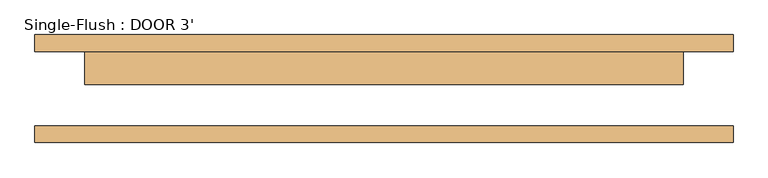
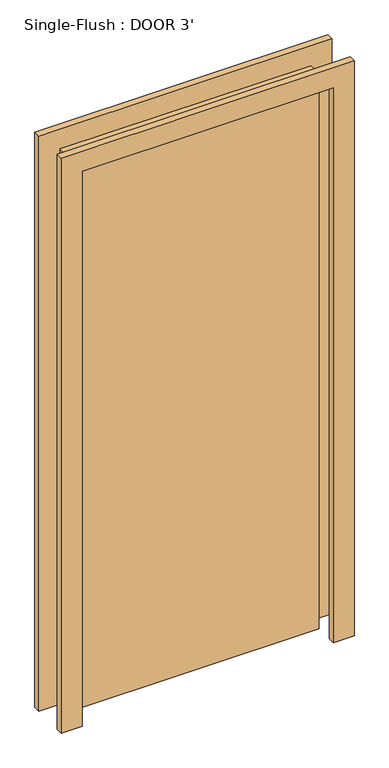
"""IFC4 building model written with IfcOpenShell, lengths in millimetres: door geometry, Single-Flush : DOOR 3'."""

from ifc_helpers import new_model, si_unit, frame, origin, origin_with_axes, place, context, project, spatial, polyline, outline, extrude, source, transform, mapped, element, save


def single_flush_door_3_e5f9f3c4(model_context):
    return source(origin(), model_context, "Body", "SweptSolid", [
        extrude(outline(polyline([(2209.8, -533.4), (0.0, -533.4), (0.0, -457.2), (2133.6, -457.2), (2133.6, 457.2), (0.0, 457.2), (0.0, 533.4), (2209.8, 533.4), (2209.8, -533.4)])), frame((0.0, 57.15, 0.0), z_axis=(0.0, 1.0, 0.0), x_axis=(0.0, 0.0, 1.0)), (0.0, 0.0, 1.0), 25.4),
        extrude(outline(polyline([(2209.8, 533.4), (2209.8, -533.4), (0.0, -533.4), (0.0, -457.2), (2133.6, -457.2), (2133.6, 457.2), (0.0, 457.2), (0.0, 533.4), (2209.8, 533.4)])), frame((0.0, -82.55, 0.0), z_axis=(0.0, 1.0, 0.0), x_axis=(0.0, 0.0, 1.0)), (0.0, 0.0, 1.0), 25.4),
        extrude(outline(polyline([(457.2, 6.35), (-457.2, 6.35), (-457.2, 57.15), (457.2, 57.15), (457.2, 6.35)])), origin_with_axes(), (0.0, 0.0, 1.0), 2133.6),
    ])


if __name__ == "__main__":
    model = new_model("IFC4")
    model_context = context("Model", 3, world=origin())
    ifc_project = project(units=[si_unit("LENGTHUNIT", "METRE", prefix="MILLI")], contexts=[model_context])
    site = spatial("IfcSite", under=ifc_project)
    building = spatial("IfcBuilding", under=site)
    placement = place(None, origin())
    single_flush_door_3_shape = single_flush_door_3_e5f9f3c4(model_context)
    element("IfcDoor", 1, ObjectType="Single-Flush : DOOR 3'", at=placement, inside=building, context=model_context, shape_type="MappedRepresentation", body=[
        mapped(single_flush_door_3_shape, transform((0.0, 0.0, 0.0), x_axis=(1.0, 0.0, 0.0), y_axis=(0.0, 1.0, 0.0), z_axis=(0.0, 0.0, 1.0))),
    ])
    save(model, "model.ifc")

# Revit data of these elements
# Type "Single-Flush : DOOR 3'"
#   Type Mark = "9"
#   Construction Type Id = "MDOOR"
#   Assembly Code = "C1020"
#   Analytic Construction = "Metal"
#   Thickness = 0' - 2"
#   Heat Transfer Coefficient (U) = 0.651978 BTU/(h·ft²·°F)
#   Height = 7' - 0"
#   Trim Projection Ext = 0' - 1"
#   Trim Projection Int = 0' - 1"
#   Trim Width = 0' - 3"
#   Width = 3' - 0"
#   Define Thermal Properties by = 1
#   Door Material = Door - Panel
#   Frame Material = Door - Frame
#   Visual Light Transmittance = 0
#   Solar Heat Gain Coefficient = 0
#   Function = (empty or 0)
#   Wall Closure = (empty or 0)
# Element 1 (IfcDoor, "Single-Flush : DOOR 3'")
#   Materials on its faces: "Door - Frame", "Door - Panel"
# Materials
#   "Door - Panel": class "Wood", colour RGB 210 159 95, transparency 0, Cost = 0
#   "Door - Frame": colour RGB 118 70 51, transparency 0, Cost = 0
